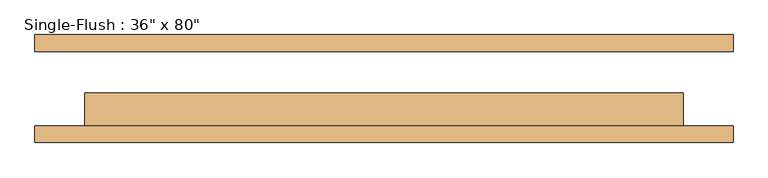
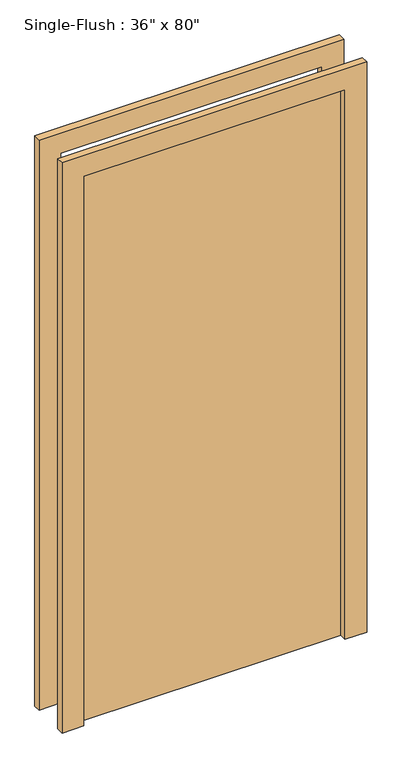
"""IFC4 building model written with IfcOpenShell, lengths in millimetres: door geometry."""

from ifc_helpers import new_model, si_unit, frame, origin, origin_with_axes, place, context, project, spatial, polyline, outline, extrude, source, transform, mapped, element, save


def door_5e62189b(model_context):
    return source(origin(), model_context, "Body", "SweptSolid", [
        extrude(outline(polyline([(2108.2, -533.4), (0.0, -533.4), (0.0, -457.2), (2032.0, -457.2), (2032.0, 457.2), (0.0, 457.2), (0.0, 533.4), (2108.2, 533.4), (2108.2, -533.4)])), frame((0.0, -82.55, 0.0), z_axis=(0.0, 1.0, 0.0), x_axis=(0.0, 0.0, 1.0)), (0.0, 0.0, 1.0), 25.4),
        extrude(outline(polyline([(2108.2, 533.4), (2108.2, -533.4), (0.0, -533.4), (0.0, -457.2), (2032.0, -457.2), (2032.0, 457.2), (0.0, 457.2), (0.0, 533.4), (2108.2, 533.4)])), frame((0.0, 57.15, 0.0), z_axis=(0.0, 1.0, 0.0), x_axis=(0.0, 0.0, 1.0)), (0.0, 0.0, 1.0), 25.4),
        extrude(outline(polyline([(457.2, -6.35), (457.2, -57.15), (-457.2, -57.15), (-457.2, -6.35), (457.2, -6.35)])), origin_with_axes(), (0.0, 0.0, 1.0), 2032.0),
    ])


if __name__ == "__main__":
    model = new_model("IFC4")
    model_context = context("Model", 3, world=origin())
    ifc_project = project(units=[si_unit("LENGTHUNIT", "METRE", prefix="MILLI")], contexts=[model_context])
    site = spatial("IfcSite", under=ifc_project)
    building = spatial("IfcBuilding", under=site)
    placement = place(None, origin())
    door_shape = door_5e62189b(model_context)
    element("IfcDoor", 1, ObjectType="Single-Flush : 36\" x 80\"", at=placement, inside=building, context=model_context, shape_type="MappedRepresentation", body=[
        mapped(door_shape, transform((0.0, 0.0, 0.0), x_axis=(1.0, 0.0, 0.0), y_axis=(0.0, 1.0, 0.0), z_axis=(0.0, 0.0, 1.0))),
    ])
    save(model, "model.ifc")

# Revit data of these elements
# Type "Single-Flush : 36\" x 80\""
#   Type Mark = "6"
#   Construction Type Id = "MDOOR"
#   Assembly Code = "C1020"
#   Analytic Construction = "Metal"
#   Thickness = 0' - 2"
#   Heat Transfer Coefficient (U) = 0.651978 BTU/(h·ft²·°F)
#   Height = 6' - 8"
#   Trim Projection Ext = 0' - 1"
#   Trim Projection Int = 0' - 1"
#   Trim Width = 0' - 3"
#   Width = 3' - 0"
#   Define Thermal Properties by = 1
#   Define Thermal Properties by = 1
#   Door Material = Door - Panel
#   Frame Material = Door - Frame
#   Visual Light Transmittance = 0
#   Solar Heat Gain Coefficient = 0
#   Function = (empty or 0)
#   Wall Closure = (empty or 0)
# Element 1 (IfcDoor, "Single-Flush : 36\" x 80\"")
#   Materials on its faces: "Door - Frame", "Door - Panel"
# Materials
#   "Door - Panel": class "Wood", colour RGB 210 159 95, transparency 0, Cost = 0
#   "Door - Frame": colour RGB 118 70 51, transparency 0, Cost = 0
